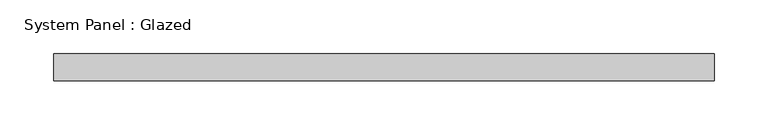
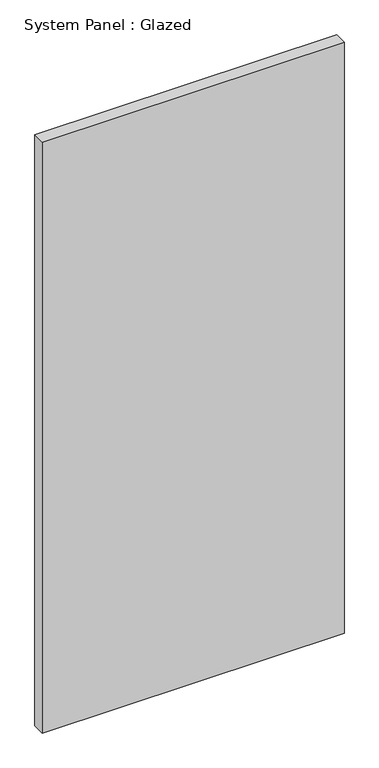
"""IFC4 building model written with IfcOpenShell, lengths in millimetres: plate geometry, System Panel : Glazed."""

from ifc_helpers import new_model, si_unit, origin, origin_with_axes, place, context, project, spatial, polyline, outline, extrude, source, transform, mapped, element, save


def system_panel_glazed_e0225be8(model_context):
    return source(origin(), model_context, "Body", "SweptSolid", [
        extrude(outline(polyline([(307.975, 19.05), (-307.975, 19.05), (-307.975, 44.45), (307.975, 44.45), (307.975, 19.05)])), origin_with_axes(), (0.0, 0.0, 1.0), 1274.8499484),
    ])


if __name__ == "__main__":
    model = new_model("IFC4")
    model_context = context("Model", 3, world=origin())
    ifc_project = project(units=[si_unit("LENGTHUNIT", "METRE", prefix="MILLI")], contexts=[model_context])
    site = spatial("IfcSite", under=ifc_project)
    building = spatial("IfcBuilding", under=site)
    placement = place(None, origin())
    system_panel_glazed_shape = system_panel_glazed_e0225be8(model_context)
    element("IfcPlate", 1, ObjectType="System Panel : Glazed", at=placement, inside=building, context=model_context, shape_type="MappedRepresentation", body=[
        mapped(system_panel_glazed_shape, transform((0.0, 0.0, 0.0), x_axis=(1.0, 0.0, 0.0), y_axis=(0.0, 1.0, 0.0), z_axis=(0.0, 0.0, 1.0))),
    ])
    save(model, "model.ifc")

# Revit data of these elements
# Type "System Panel : Glazed"
#   Construction Type Id = "GSP4R"
#   Analytic Construction = "1/8 in Pilkington single glazing"
#   Visual Light Transmittance = 0.9
#   Solar Heat Gain Coefficient = 0.86
#   Heat Transfer Coefficient (U) = 1.18115 BTU/(h·ft²·°F)
#   Define Thermal Properties by = 1
# Element 1 (IfcPlate, "System Panel : Glazed")
#   Materials on its faces: "Glass"
# Materials
#   "Glass": class "Glass", colour RGB 0 128 192, transparency 0.75, Description = "Soda Lime Glass", Cost = 0
